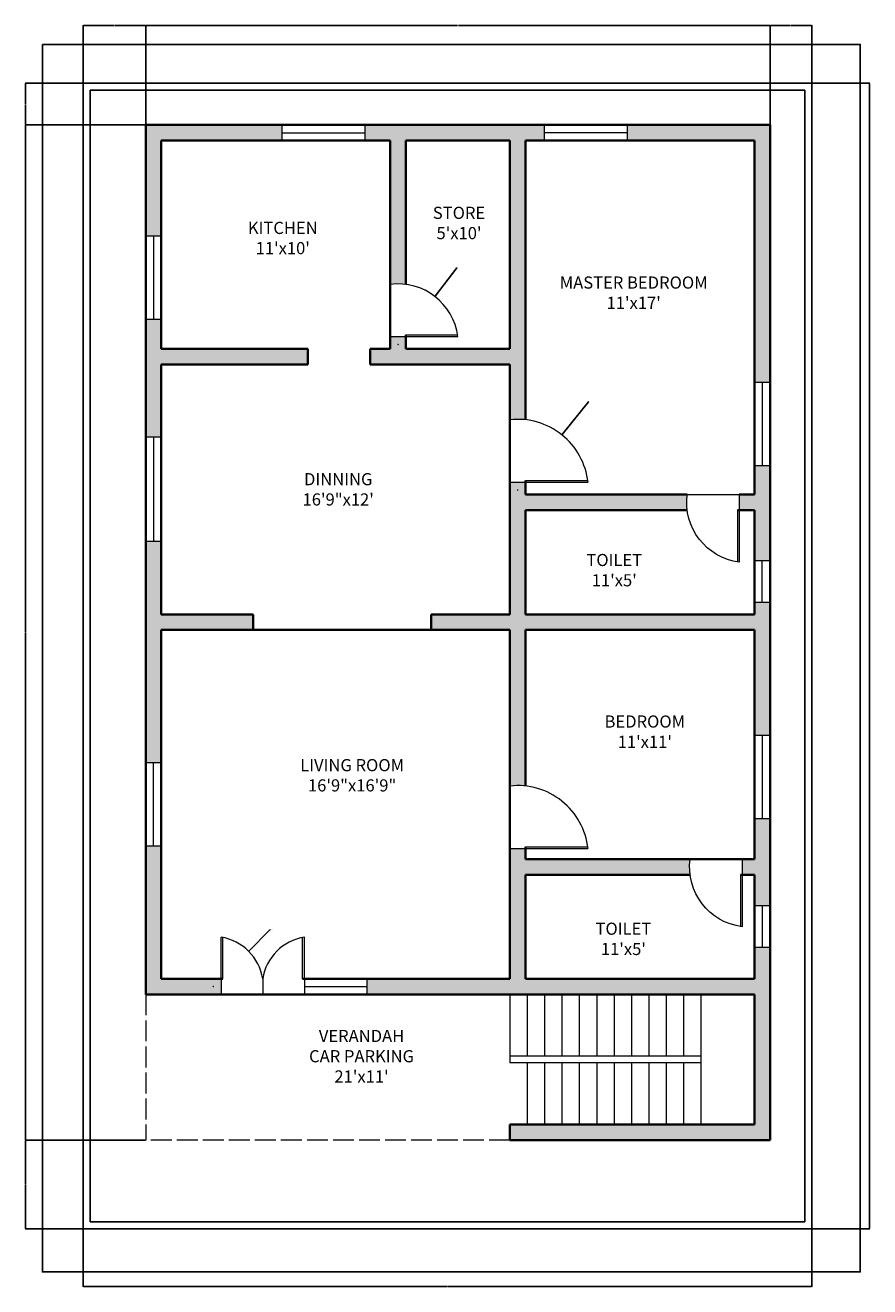
# Model space of a CAD drawing. Units: inches. Extents: x 4948 to 20975, y 6797 to 20508.
# Tile 1 of 5: x 4948 to 5435, y 6797 to 7524. Entities that reach past the tile are written whole.
import ezdxf

# ---------------------------------------------------------------- set-up
doc = ezdxf.new("R2010")
doc.units = ezdxf.units.IN
doc.linetypes.add('ACAD_ISO02W100', pattern=[15, 12, -3])
for name, color, linetype, lineweight in [('A-ANNO-DIMS', 2, 'Continuous', 18), ('A-ANNO-TTLB', 7, 'Continuous', 25), ('A-AREA-IDEN', 7, 'Continuous', 25), ('A-DOOR', 3, 'Continuous', 18), ('A-FLOR-OVHD', 8, 'ACAD_ISO02W100', 18), ('A-FLOR-STRS', 7, 'Continuous', 18), ('A-GLAZ', 4, 'Continuous', 18), ('A-WALL', 7, 'Continuous', 35), ('C-PROP', 7, 'Continuous', 25)]:
    doc.layers.add(name, color=color, linetype=linetype, lineweight=lineweight)
doc.layers.add('A-WALL-PATT', color=18, linetype='Continuous', lineweight=13, true_color=0x000000)
doc.styles.get("Standard").update_dxf_attribs({"font": 'times.ttf'})
doc.dimstyles.get("Standard").update_dxf_attribs({"dimtxt": 0.18, "dimasz": 0.18, "dimexe": 0.18, "dimexo": 0.0625, "dimgap": 0.09, "dimtad": 0, "dimtih": 1, "dimtoh": 1, "dimdec": 4, "dimzin": 0, "dimdsep": 46, "dimtxsty": 'Standard', "dimcen": 0.09, "dimadec": 0, "dimazin": 0, "dimtfac": 1, "dimtdec": 4, "dimtofl": 0, "dimtmove": 0, "dimatfit": 3, "dimfxl": 1, "dimtolj": 1, "dimtzin": 0, "dimarcsym": 0})

# ---------------------------------------------------------------- blocks, each defined once
blk = doc.blocks.new('DOOR-SINGLE-36IN')
for p, q in [((9, 1), (45, 1)), ((0, 0), (9, 0)), ((9, 0), (45, 0))]:
    blk.add_line(p, q)
blk.add_arc((4.5, -4.5), 40.75, 6.34019, 96.34019)
blk = doc.blocks.new('DOOR-SINGLE-30IN')
for p, q in [((0, 0), (9, 0)), ((9, 1), (39, 1)), ((9, 0), (39, 0))]:
    blk.add_line(p, q)
blk.add_arc((4.5, -4.5), 34.79, 7.43141, 97.43141)
blk = doc.blocks.new('DOOR-DOUBLE-48IN')
for p, q in [((0, 9), (0, 33)), ((1, 9), (1, 33)), ((47, 9), (47, 33)), ((48, 9), (48, 33)), ((0, 9), (0, 0)), ((24, 9), (24, 0)), ((48, 9), (48, 0))]:
    blk.add_line(p, q)
for centre, start, end in [((-4.5, 4.5), 8.97263, 81.02737), ((52.5, 4.5), 98.97263, 171.02737)]:
    blk.add_arc(centre, 28.85, start, end)
blk = doc.blocks.new('WIN-48IN')
for p, q in [((0, 0), (0, 9)), ((48, 0), (48, 9)), ((0, 4.5), (48, 4.5))]:
    blk.add_line(p, q)
blk = doc.blocks.new('WIN-24IN')
for p, q in [((0, 24), (9, 24)), ((4.5, 0), (4.5, 24)), ((0, 0), (9, 0))]:
    blk.add_line(p, q)
blk = doc.blocks.new('WIN-SIDELIGHT-36IN')
for p, q in [((36, 9), (36, 0)), ((0, 4.5), (36, 4.5))]:
    blk.add_line(p, q)
blk = doc.blocks.new('WIN-60IN')
for p, q in [((9, 60), (0, 60)), ((4.5, 60), (4.5, 0)), ((9, 0), (0, 0))]:
    blk.add_line(p, q)
blk = doc.blocks.new('STAIR-RETURN-110IN')
for p, q in [((0, 75), (0, 35.5)), ((10, 75), (10, 39.5)), ((20, 75), (20, 39.5)), ((30, 75), (30, 39.5)), ((40, 75), (40, 39.5)), ((50, 75), (50, 39.5)), ((60, 75), (60, 39.5)), ((70, 75), (70, 39.5)), ((80, 75), (80, 39.5)), ((90, 75), (90, 39.5)), ((100, 75), (100, 39.5)), ((110, 75), (110, 0)), ((110, 39.5), (0, 39.5)), ((110, 35.5), (0, 35.5)), ((10, 35.5), (10, 0)), ((20, 35.5), (20, 0)), ((30, 35.5), (30, 0)), ((40, 35.5), (40, 0)), ((50, 35.5), (50, 0)), ((60, 35.5), (60, 0)), ((70, 35.5), (70, 0)), ((80, 35.5), (80, 0)), ((90, 35.5), (90, 0)), ((100, 35.5), (100, 0))]:
    blk.add_line(p, q)
blk = doc.blocks.new('*D25')
at = {"layer": 'A-ANNO-DIMS', "color": 0, "lineweight": -2, "transparency": 16777216}
for p, q in [((4981.22, 6830.38), (4981.22, 6797.01)), ((5401.22, 6830.38), (5401.22, 6797.01)), ((4981.4, 6797.19), (5190.94, 6797.19)), ((5401.04, 6797.19), (5191.5, 6797.19))]:
    blk.add_line(p, q, dxfattribs=at)
at = {"layer": 'A-ANNO-DIMS', "color": 0, "transparency": 16777216}
for points in [[(4981.4, 6797.22), (4981.4, 6797.16), (4981.22, 6797.19)], [(5401.04, 6797.22), (5401.04, 6797.16), (5401.22, 6797.19)]]:
    blk.add_solid(points, dxfattribs=at)
at = {"layer": 'Defpoints', "color": 0, "transparency": 16777216}
for p in [(4981.22, 6830.44), (5401.22, 6830.44), (5401.22, 6797.19)]:
    blk.add_point(p, dxfattribs=at)
at = {"layer": 'A-ANNO-DIMS', "color": 0, "transparency": 16777216, "insert": (5191.22, 6797.19), "char_height": 0.18, "attachment_point": 5}
blk.add_mtext('\\A1;420', dxfattribs=at)
blk = doc.blocks.new('*D26')
at = {"layer": 'A-ANNO-DIMS', "color": 0, "lineweight": -2, "transparency": 16777216}
for p, q in [((5401.28, 7490.44), (5434.65, 7490.44)), ((5434.47, 7490.26), (5434.47, 7160.63)), ((5434.47, 6830.62), (5434.47, 7160.26)), ((5401.28, 6830.44), (5434.65, 6830.44))]:
    blk.add_line(p, q, dxfattribs=at)
at = {"layer": 'A-ANNO-DIMS', "color": 0, "transparency": 16777216}
for points in [[(5434.44, 7490.26), (5434.5, 7490.26), (5434.47, 7490.44)], [(5434.44, 6830.62), (5434.5, 6830.62), (5434.47, 6830.44)]]:
    blk.add_solid(points, dxfattribs=at)
at = {"layer": 'Defpoints', "color": 0, "transparency": 16777216}
for p in [(5401.22, 7490.44), (5434.47, 7490.44), (5401.22, 6830.44)]:
    blk.add_point(p, dxfattribs=at)
at = {"layer": 'A-ANNO-DIMS', "color": 0, "transparency": 16777216, "insert": (5434.47, 7160.44), "char_height": 0.18, "attachment_point": 5}
blk.add_mtext('\\A1;660', dxfattribs=at)
blk = doc.blocks.new('*D27')
at = {"layer": 'A-ANNO-DIMS', "color": 0, "lineweight": -2, "transparency": 16777216}
for p, q in [((5017.22, 7466.51), (5017.22, 7523.87)), ((5017.4, 7523.69), (5196.94, 7523.69)), ((5377.04, 7523.69), (5197.5, 7523.69)), ((5377.22, 7466.51), (5377.22, 7523.87))]:
    blk.add_line(p, q, dxfattribs=at)
at = {"layer": 'A-ANNO-DIMS', "color": 0, "transparency": 16777216}
for points in [[(5017.4, 7523.72), (5017.4, 7523.66), (5017.22, 7523.69)], [(5377.04, 7523.72), (5377.04, 7523.66), (5377.22, 7523.69)]]:
    blk.add_solid(points, dxfattribs=at)
at = {"layer": 'Defpoints', "color": 0, "transparency": 16777216}
for p in [(5377.22, 7523.69), (5017.22, 7466.44), (5377.22, 7466.44)]:
    blk.add_point(p, dxfattribs=at)
at = {"layer": 'A-ANNO-DIMS', "color": 0, "transparency": 16777216, "insert": (5197.22, 7523.69), "char_height": 0.18, "attachment_point": 5}
blk.add_mtext('\\A1;360', dxfattribs=at)
blk = doc.blocks.new('*D28')
at = {"layer": 'A-ANNO-DIMS', "color": 0, "lineweight": -2, "transparency": 16777216}
for p, q in [((5017.16, 7466.44), (4947.79, 7466.44)), ((4947.97, 7466.26), (4947.97, 7174.13)), ((4947.97, 6881.62), (4947.97, 7173.76)), ((5017.16, 6881.44), (4947.79, 6881.44))]:
    blk.add_line(p, q, dxfattribs=at)
at = {"layer": 'A-ANNO-DIMS', "color": 0, "transparency": 16777216}
for points in [[(4947.94, 7466.26), (4948, 7466.26), (4947.97, 7466.44)], [(4947.94, 6881.62), (4948, 6881.62), (4947.97, 6881.44)]]:
    blk.add_solid(points, dxfattribs=at)
at = {"layer": 'Defpoints', "color": 0, "transparency": 16777216}
for p in [(4947.97, 7466.44), (5017.22, 7466.44), (5017.22, 6881.44)]:
    blk.add_point(p, dxfattribs=at)
at = {"layer": 'A-ANNO-DIMS', "color": 0, "transparency": 16777216, "insert": (4947.97, 7173.94), "char_height": 0.18, "attachment_point": 5}
blk.add_mtext('\\A1;585', dxfattribs=at)
blk = doc.blocks.new('*D29')
at = {"layer": 'A-ANNO-DIMS', "color": 0, "lineweight": -2, "transparency": 16777216}
for p, q in [((4981.22, 7490.51), (4981.22, 7523.87)), ((4981.4, 7523.69), (4999.01, 7523.69)), ((5017.04, 7523.69), (4999.43, 7523.69)), ((5017.22, 7466.51), (5017.22, 7523.87))]:
    blk.add_line(p, q, dxfattribs=at)
at = {"layer": 'A-ANNO-DIMS', "color": 0, "transparency": 16777216}
for points in [[(4981.4, 7523.72), (4981.4, 7523.66), (4981.22, 7523.69)], [(5017.04, 7523.72), (5017.04, 7523.66), (5017.22, 7523.69)]]:
    blk.add_solid(points, dxfattribs=at)
at = {"layer": 'Defpoints', "color": 0, "transparency": 16777216}
for p in [(5017.22, 7523.69), (4981.22, 7490.44), (5017.22, 7466.44)]:
    blk.add_point(p, dxfattribs=at)
at = {"layer": 'A-ANNO-DIMS', "color": 0, "transparency": 16777216, "insert": (4999.22, 7523.69), "char_height": 0.18, "attachment_point": 5}
blk.add_mtext('\\A1;36', dxfattribs=at)
blk = doc.blocks.new('*D30')
at = {"layer": 'A-ANNO-DIMS', "color": 0, "lineweight": -2, "transparency": 16777216}
for p, q in [((5377.22, 7466.51), (5377.22, 7523.87)), ((5377.4, 7523.69), (5389, 7523.69)), ((5401.04, 7523.69), (5389.43, 7523.69)), ((5401.22, 7490.51), (5401.22, 7523.87))]:
    blk.add_line(p, q, dxfattribs=at)
at = {"layer": 'A-ANNO-DIMS', "color": 0, "transparency": 16777216}
for points in [[(5377.4, 7523.72), (5377.4, 7523.66), (5377.22, 7523.69)], [(5401.04, 7523.72), (5401.04, 7523.66), (5401.22, 7523.69)]]:
    blk.add_solid(points, dxfattribs=at)
at = {"layer": 'Defpoints', "color": 0, "transparency": 16777216}
for p in [(5401.22, 7523.69), (5401.22, 7490.44), (5377.22, 7466.44)]:
    blk.add_point(p, dxfattribs=at)
at = {"layer": 'A-ANNO-DIMS', "color": 0, "transparency": 16777216, "insert": (5389.22, 7523.69), "char_height": 0.18, "attachment_point": 5}
blk.add_mtext('\\A1;24', dxfattribs=at)
blk = doc.blocks.new('*D31')
at = {"layer": 'A-ANNO-DIMS', "color": 0, "lineweight": -2, "transparency": 16777216}
for p, q in [((4981.156446, 7490.444038), (4947.788946, 7490.444038)), ((4947.968946, 7490.264038), (4947.968946, 7478.624038)), ((4947.968946, 7466.624038), (4947.968946, 7478.264038)), ((5017.156446, 7466.444038), (4947.788946, 7466.444038))]:
    blk.add_line(p, q, dxfattribs=at)
at = {"layer": 'A-ANNO-DIMS', "color": 0, "transparency": 16777216}
for points in [[(4947.938946, 7490.264038), (4947.998946, 7490.264038), (4947.968946, 7490.444038)], [(4947.938946, 7466.624038), (4947.998946, 7466.624038), (4947.968946, 7466.444038)]]:
    blk.add_solid(points, dxfattribs=at)
at = {"layer": 'Defpoints', "color": 0, "transparency": 16777216}
for p in [(4981.218946, 7490.444038), (4947.968946, 7466.444038), (5017.218946, 7466.444038)]:
    blk.add_point(p, dxfattribs=at)
at = {"layer": 'A-ANNO-DIMS', "color": 0, "transparency": 16777216, "insert": (4947.968946, 7478.444038), "char_height": 0.18, "attachment_point": 5}
blk.add_mtext('\\A1;24', dxfattribs=at)
blk = doc.blocks.new('*D32')
at = {"layer": 'A-ANNO-DIMS', "color": 0, "lineweight": -2, "transparency": 16777216}
for p, q in [((5017.16, 6881.44), (4947.79, 6881.44)), ((4947.97, 6881.26), (4947.97, 6856.13)), ((4947.97, 6830.62), (4947.97, 6855.76)), ((4981.16, 6830.44), (4947.79, 6830.44))]:
    blk.add_line(p, q, dxfattribs=at)
at = {"layer": 'A-ANNO-DIMS', "color": 0, "transparency": 16777216}
for points in [[(4947.94, 6881.26), (4948, 6881.26), (4947.97, 6881.44)], [(4947.94, 6830.62), (4948, 6830.62), (4947.97, 6830.44)]]:
    blk.add_solid(points, dxfattribs=at)
at = {"layer": 'Defpoints', "color": 0, "transparency": 16777216}
for p in [(4947.97, 6881.44), (5017.22, 6881.44), (4981.22, 6830.44)]:
    blk.add_point(p, dxfattribs=at)
at = {"layer": 'A-ANNO-DIMS', "color": 0, "transparency": 16777216, "insert": (4947.97, 6855.94), "char_height": 0.18, "attachment_point": 5}
blk.add_mtext('\\A1;51', dxfattribs=at)
blk = doc.blocks.new('*D87')
at = {"layer": 'A-ANNO-DIMS', "color": 0, "lineweight": -2, "transparency": 16777216}
for p, q in [((5272.45, 7306.96), (5257.29, 7288.01)), ((5272.63, 7306.96), (5272.45, 7306.96)), ((5231.63, 7256.05), (5231.81, 7256.05)), ((5231.72, 7255.96), (5231.72, 7256.14))]:
    blk.add_line(p, q, dxfattribs=at)
at = {"layer": 'A-ANNO-DIMS', "color": 0, "transparency": 16777216}
blk.add_solid([(5257.26, 7288.03), (5257.31, 7287.99), (5257.18, 7287.87)], dxfattribs=at)
at = {"layer": 'Defpoints', "color": 0, "transparency": 16777216}
for p in [(5257.18, 7287.87), (5231.72, 7256.05)]:
    blk.add_point(p, dxfattribs=at)
at = {"layer": 'A-ANNO-DIMS', "color": 0, "transparency": 16777216, "insert": (5273.29, 7306.96), "char_height": 0.18, "attachment_point": 5}
blk.add_mtext('\\A1;2X R40.75', dxfattribs=at)
blk = doc.blocks.new('*D88')
at = {"layer": 'A-ANNO-DIMS', "color": 0, "lineweight": -2, "transparency": 16777216}
for p, q in [((5196.66, 7384.13), (5184.04, 7367.73)), ((5196.84, 7384.13), (5196.66, 7384.13)), ((5162.63, 7340.01), (5162.81, 7340.01)), ((5162.72, 7339.92), (5162.72, 7340.1))]:
    blk.add_line(p, q, dxfattribs=at)
at = {"layer": 'A-ANNO-DIMS', "color": 0, "transparency": 16777216}
blk.add_solid([(5184.02, 7367.75), (5184.07, 7367.71), (5183.93, 7367.59)], dxfattribs=at)
at = {"layer": 'Defpoints', "color": 0, "transparency": 16777216}
for p in [(5183.93, 7367.59), (5162.72, 7340.01)]:
    blk.add_point(p, dxfattribs=at)
at = {"layer": 'A-ANNO-DIMS', "color": 0, "transparency": 16777216, "insert": (5197.31, 7384.13), "char_height": 0.18, "attachment_point": 5}
blk.add_mtext('\\A1;R34.79', dxfattribs=at)
blk = doc.blocks.new('*D89')
at = {"layer": 'A-ANNO-DIMS', "color": 0, "lineweight": -2, "transparency": 16777216}
for p, q in [((5088.83, 7002.59), (5076.71, 6990.47)), ((5089.01, 7002.59), (5088.83, 7002.59)), ((5056.09, 6969.94), (5056.27, 6969.94)), ((5056.18, 6969.85), (5056.18, 6970.03))]:
    blk.add_line(p, q, dxfattribs=at)
at = {"layer": 'A-ANNO-DIMS', "color": 0, "transparency": 16777216}
blk.add_solid([(5076.69, 6990.49), (5076.73, 6990.45), (5076.58, 6990.35)], dxfattribs=at)
at = {"layer": 'Defpoints', "color": 0, "transparency": 16777216}
for p in [(5076.58, 6990.35), (5056.18, 6969.94)]:
    blk.add_point(p, dxfattribs=at)
at = {"layer": 'A-ANNO-DIMS', "color": 0, "transparency": 16777216, "insert": (5089.73, 7002.59), "char_height": 0.18, "attachment_point": 5}
blk.add_mtext('\\A1;2X R28.853', dxfattribs=at)

msp = doc.modelspace()

# ---------------------------------------------------------------- hatches: boundary and pattern name
at = {"layer": 'A-WALL-PATT'}
h = msp.add_hatch(color=256, dxfattribs=at)
h.dxf.hatch_style = 1
h.paths.add_polyline_path([(5095.8403, 7466.444), (5017.2189, 7466.444), (5017.2189, 7402.5352), (5026.2189, 7402.5352), (5026.2189, 7457.444), (5095.8403, 7457.444)])
h.paths.add_polyline_path([(5246.8789, 7466.444), (5143.8403, 7466.444), (5143.8403, 7457.444), (5158.2189, 7457.444), (5158.2189, 7374.5094, -0.06494234), (5167.2189, 7374.5094), (5167.2189, 7457.444), (5227.2189, 7457.444), (5227.2189, 7337.444), (5167.2189, 7337.444), (5167.2189, 7344.5094), (5158.2189, 7344.5094), (5158.2189, 7337.444), (5146.6872, 7337.444), (5146.6872, 7328.444), (5227.2189, 7328.444), (5227.2189, 7296.5526, -0.05538514), (5236.2189, 7296.5526), (5236.2189, 7328.444), (5236.2189, 7457.444), (5246.8789, 7457.444)])
h.paths.add_polyline_path([(5377.2189, 7466.444), (5294.8789, 7466.444), (5294.8789, 7457.444), (5368.2189, 7457.444), (5368.2189, 7318.1488), (5377.2189, 7318.1488)])
h.paths.add_polyline_path([(5026.2189, 7328.444), (5110.6872, 7328.444), (5110.6872, 7337.444), (5026.2189, 7337.444), (5026.2189, 7354.5352), (5017.2189, 7354.5352), (5017.2189, 7286.444), (5026.2189, 7286.444)])
h.paths.add_polyline_path([(5377.2189, 7191.5422), (5368.2189, 7191.5422), (5368.2189, 7184.444), (5236.2189, 7184.444), (5236.2189, 7244.444), (5329.4566, 7244.444, -0.06494234), (5329.4566, 7253.444), (5236.2189, 7253.444), (5236.2189, 7260.5526), (5227.2189, 7260.5526), (5227.2189, 7244.444), (5227.2189, 7184.444), (5181.8226, 7184.444), (5181.8226, 7175.444), (5227.2189, 7175.444), (5227.2189, 7085.5219, -0.05538514), (5236.2189, 7085.5219), (5236.2189, 7175.444), (5368.2189, 7175.444), (5368.2189, 7114.8955), (5377.2189, 7114.8955)])
h.paths.add_polyline_path([(5377.2189, 7270.1488), (5368.2189, 7270.1488), (5368.2189, 7253.444), (5359.4566, 7253.444), (5359.4566, 7244.444), (5368.2189, 7244.444), (5368.2189, 7215.5422), (5377.2189, 7215.5422)])
h.paths.add_polyline_path([(5377.2189, 7066.8955), (5368.2189, 7066.8955), (5368.2189, 7043.444), (5361.0558, 7043.444), (5361.0558, 7034.444), (5368.2189, 7034.444), (5368.2189, 7016.444), (5377.2189, 7016.444)])
h.paths.add_polyline_path([(5377.2189, 6992.444), (5368.2189, 6992.444), (5368.2189, 6974.444), (5236.2189, 6974.444), (5236.2189, 7034.444), (5331.0558, 7034.444, -0.06494234), (5331.0558, 7043.444), (5236.2189, 7043.444), (5236.2189, 7049.5219), (5227.2189, 7049.5219), (5227.2189, 6974.444), (5144.6817, 6974.444), (5144.6817, 6965.444), (5227.2189, 6965.444), (5236.2189, 6965.444), (5368.2189, 6965.444), (5368.2189, 6890.444), (5227.2189, 6890.444), (5227.2189, 6881.444), (5377.2189, 6881.444)])
h.paths.add_polyline_path([(5060.6817, 6974.444), (5026.2189, 6974.444), (5026.2189, 7050.944), (5017.2189, 7050.944), (5017.2189, 6965.444), (5026.2189, 6965.444), (5060.6817, 6965.444)])
h.paths.add_polyline_path([(5026.2189, 7175.444), (5079.1853, 7175.444), (5079.1853, 7184.444), (5026.2189, 7184.444), (5026.2189, 7226.444), (5017.2189, 7226.444), (5017.2189, 7098.944), (5026.2189, 7098.944)])

# ---------------------------------------------------------------- linework, layer by layer
at = {"layer": 'A-ANNO-TTLB'}
msp.add_lwpolyline([(4957.7293, 7512.8595), (5429.1896, 7512.8595), (5429.1896, 6805.5342), (4957.7293, 6805.5342)], close=True, dxfattribs=at)
at = {"layer": 'A-DOOR'}
msp.add_line((5329.4566, 7253.444), (5359.4566, 7253.444), dxfattribs=at)
at = {"layer": 'A-FLOR-OVHD'}
for p in [(5017.2189, 6965.444), (5227.2189, 6881.444)]:
    msp.add_line(p, (5017.2189, 6881.444), dxfattribs=at)
at = {"layer": 'A-WALL'}
for p, q in [((5017.2189, 6965.444), (5017.2189, 7466.444)), ((5017.2189, 7466.444), (5377.2189, 7466.444)), ((5377.2189, 7466.444), (5377.2189, 6881.444)), ((5026.2189, 7457.444), (5158.2189, 7457.444)), ((5026.2189, 7337.444), (5026.2189, 7457.444)), ((5158.2189, 7337.444), (5158.2189, 7457.444)), ((5167.2189, 7457.444), (5227.2189, 7457.444)), ((5167.2189, 7374.5094), (5167.2189, 7457.444)), ((5227.2189, 7337.444), (5227.2189, 7457.444)), ((5236.2189, 7328.444), (5236.2189, 7457.444)), ((5236.2189, 7457.444), (5368.2189, 7457.444)), ((5368.2189, 7457.444), (5368.2189, 7253.444)), ((5167.2189, 7337.444), (5167.2189, 7345.5094)), ((5026.2189, 7337.444), (5110.6872, 7337.444)), ((5110.6872, 7337.444), (5110.6872, 7328.444)), ((5146.6872, 7337.444), (5146.6872, 7328.444)), ((5146.6872, 7337.444), (5158.2189, 7337.444)), ((5167.2189, 7337.444), (5227.2189, 7337.444)), ((5026.2189, 7328.444), (5110.6872, 7328.444)), ((5026.2189, 7184.444), (5026.2189, 7328.444)), ((5146.6872, 7328.444), (5227.2189, 7328.444)), ((5227.2189, 7328.444), (5227.2189, 7244.444)), ((5236.2189, 7328.444), (5236.2189, 7296.5526)), ((5236.2189, 7261.5526), (5236.2189, 7253.444)), ((5236.2189, 7253.444), (5329.4566, 7253.444)), ((5359.4566, 7253.444), (5368.2189, 7253.444)), ((5227.2189, 7244.444), (5227.2189, 7184.444)), ((5236.2189, 7244.444), (5329.4566, 7244.444)), ((5236.2189, 7244.444), (5236.2189, 7184.444)), ((5358.4566, 7244.444), (5368.2189, 7244.444)), ((5368.2189, 7244.444), (5368.2189, 7184.444)), ((5026.2189, 7184.444), (5079.1853, 7184.444)), ((5079.1853, 7175.444), (5079.1853, 7184.444)), ((5181.8226, 7175.444), (5181.8226, 7184.444)), ((5181.8226, 7184.444), (5227.2189, 7184.444)), ((5236.2189, 7184.444), (5368.2189, 7184.444)), ((5026.2189, 7175.444), (5079.1853, 7175.444)), ((5026.2189, 6974.444), (5026.2189, 7175.444)), ((5079.1853, 7175.444), (5181.8226, 7175.444)), ((5181.8226, 7175.444), (5227.2189, 7175.444)), ((5227.2189, 7175.444), (5227.2189, 6974.444)), ((5236.2189, 7175.444), (5236.2189, 7085.5219)), ((5236.2189, 7175.444), (5368.2189, 7175.444)), ((5368.2189, 7175.444), (5368.2189, 7043.444)), ((5236.2189, 7050.5219), (5236.2189, 7043.444)), ((5236.2189, 7043.444), (5368.2189, 7043.444)), ((5236.2189, 7034.444), (5331.0558, 7034.444)), ((5236.2189, 7034.444), (5236.2189, 6974.444)), ((5360.0558, 7034.444), (5368.2189, 7034.444)), ((5368.2189, 7034.444), (5368.2189, 6974.444)), ((5026.2189, 6974.444), (5061.6817, 6974.444)), ((5107.6817, 6974.444), (5227.2189, 6974.444)), ((5236.2189, 6974.444), (5368.2189, 6974.444)), ((5026.2189, 6965.444), (5017.2189, 6965.444)), ((5026.2189, 6965.444), (5227.2189, 6965.444)), ((5227.2189, 6965.444), (5236.2189, 6965.444)), ((5236.2189, 6965.444), (5368.2189, 6965.444)), ((5368.2189, 6965.444), (5368.2189, 6890.444)), ((5368.2189, 6890.444), (5227.2189, 6890.444)), ((5227.2189, 6890.444), (5227.2189, 6881.444)), ((5377.2189, 6881.444), (5227.2189, 6881.444))]:
    msp.add_line(p, q, dxfattribs=at)
at = {"layer": 'C-PROP'}
for p, q in [((4981.2189, 7490.444), (5401.2189, 7490.444)), ((4981.2189, 6830.444), (4981.2189, 7490.444)), ((5401.2189, 7490.444), (5401.2189, 6830.444)), ((4985.2189, 7486.444), (5397.2189, 7486.444)), ((4985.2189, 6834.444), (4985.2189, 7486.444)), ((5397.2189, 7486.444), (5397.2189, 6834.444)), ((5397.2189, 6834.444), (4985.2189, 6834.444)), ((5401.2189, 6830.444), (4981.2189, 6830.444))]:
    msp.add_line(p, q, dxfattribs=at)

# ---------------------------------------------------------------- block references
at = {"layer": 'A-DOOR'}
for name, p in [('DOOR-SINGLE-30IN', (5158.219, 7344.509)), ('DOOR-SINGLE-36IN', (5227.219, 7260.553)), ('DOOR-SINGLE-36IN', (5227.219, 7049.5222)), ('DOOR-DOUBLE-48IN', (5060.682, 6965.444))]:
    msp.add_blockref(name, p, dxfattribs=at)
at = {"layer": 'A-DOOR', "extrusion": (0, 0, -1), "zscale": -1}
for p, rotation in [((-5359.4571, 7253.444), 269.9999999999948), ((-5361.0562, 7043.444), 269.9999999999951)]:
    msp.add_blockref('DOOR-SINGLE-30IN', p, dxfattribs=dict(at, rotation=rotation))
at = {"layer": 'A-FLOR-STRS'}
msp.add_blockref('STAIR-RETURN-110IN', (5227.219, 6890.444), dxfattribs=at)
at = {"layer": 'A-GLAZ'}
for name, p in [('WIN-48IN', (5095.84, 7457.444)), ('WIN-60IN', (5017.219, 7226.444)), ('WIN-24IN', (5368.219, 7191.542)), ('WIN-SIDELIGHT-36IN', (5108.682, 6965.444))]:
    msp.add_blockref(name, p, dxfattribs=at)
for name, p, rotation in [('WIN-48IN', (5294.8792, 7466.4441), 180), ('WIN-48IN', (5017.2189, 7402.5355), 269.999999999995), ('WIN-48IN', (5368.2189, 7318.1491), 269.9999999999816), ('WIN-48IN', (5368.2189, 7114.8958), 269.9999999999971), ('WIN-48IN', (5026.219, 7050.9437), 89.99999999999083), ('WIN-24IN', (5377.2189, 7016.4442), 180)]:
    msp.add_blockref(name, p, dxfattribs=dict(at, rotation=rotation))

# ---------------------------------------------------------------- texts
at = {"layer": 'A-AREA-IDEN', "char_height": 7, "attachment_point": 1}
for s, width, insert in [("\\pxqc;{\\fTimes New Roman|b1|i0|c0|p18;STORE\\P5'x10'}", 45.669043, (5175.0326, 7419.2695)), ("\\pxqc;{\\fTimes New Roman|b1|i0|c0|p18;KITCHEN\\P11'x10'}", 91.794797, (5050.3561, 7410.5979)), ("\\pxqc;{\\fTimes New Roman|b1|i0|c0|p18;MASTER BEDROOM 11'x17'}", 108.235638, (5244.4496, 7379.1063)), ('\\pxqc;{\\fTimes New Roman|b1|i0|c0|p18;DINNING\\P16\'9"x12\'}', 128.330031, (5064.0518, 7265.8125)), ("\\pxqc;{\\fTimes New Roman|b1|i0|c0|p18;TOILET\\P11'x5'}", 86.771181, (5243.9879, 7219.2596)), ("\\pxqc;{\\fTimes New Roman|b1|i0|c0|p18;BEDROOM\\P11'x11'}", 109.747903, (5250.1091, 7126.191)), ('\\pxqc;{\\fTimes New Roman|b1|i0|c0|p18;LIVING ROOM\\P16\'9"x16\'9"}', 113.406157, (5079.5425, 7101.0564)), ("\\pxqc;{\\fTimes New Roman|b1|i0|c0|p18;TOILET\\P11'x5'}", 85.969216, (5249.6482, 7006.8141)), ("\\pxqc;{\\fTimes New Roman|b1|i0|c0|p18;VERANDAH\\PCAR PARKING\\P21'x11'}", 117.979027, (5082.671, 6945.0119))]:
    msp.add_mtext_dynamic_manual_height_columns(s, width=width, gutter_width=12.5, heights=[0], dxfattribs=dict(at, insert=insert))

# ---------------------------------------------------------------- dimensions: what is measured, and where the dimension line sits
at = {"layer": 'A-ANNO-DIMS'}
for base, p1, p2, picture, middle in [((5017.2189, 7523.694), (4981.2189, 7490.444), (5017.2189, 7466.444), '*D29', (4999.2189, 7523.694)), ((5377.2189, 7523.694), (5017.2189, 7466.444), (5377.2189, 7466.444), '*D27', (5197.2189, 7523.694)), ((5401.2189, 7523.694), (5377.2189, 7466.444), (5401.2189, 7490.444), '*D30', (5389.2189, 7523.694)), ((5401.2189, 6797.194), (4981.2189, 6830.444), (5401.2189, 6830.444), '*D25', (5191.2189, 6797.194))]:
    dim = msp.add_linear_dim(base=base, p1=p1, p2=p2, dimstyle='Standard', override={"dimdec": 0, "dimlfac": 1, "dimrnd": 0, "dimzin": 0, "dimdsep": 46, "dimlunit": 2}, dxfattribs=at)
    dim.commit()
    dim.dimension.update_dxf_attribs({"geometry": picture, "text_midpoint": middle})
for base, p1, p2, picture, middle in [((4947.9689, 7466.444), (4981.2189, 7490.444), (5017.2189, 7466.444), '*D31', (4947.9689, 7478.444)), ((5434.4689, 7490.444), (5401.2189, 6830.444), (5401.2189, 7490.444), '*D26', (5434.4689, 7160.444)), ((4947.9689, 7466.444), (5017.2189, 6881.444), (5017.2189, 7466.444), '*D28', (4947.9689, 7173.944)), ((4947.9689, 6881.444), (4981.2189, 6830.444), (5017.2189, 6881.444), '*D32', (4947.9689, 6855.944))]:
    dim = msp.add_linear_dim(base=base, p1=p1, p2=p2, angle=90, dimstyle='Standard', override={"dimdec": 0, "dimlfac": 1, "dimrnd": 0, "dimzin": 0, "dimdsep": 46, "dimlunit": 2}, dxfattribs=at)
    dim.commit()
    dim.dimension.update_dxf_attribs({"geometry": picture, "text_midpoint": middle})
dim = msp.add_radius_dim(center=(5162.7189, 7340.0094), mpoint=(5183.9319, 7367.5868), dimstyle='Standard', override={"dimdec": 2, "dimlfac": 1, "dimrnd": 0, "dimzin": 0, "dimdsep": 46, "dimlunit": 2}, dxfattribs=at)
dim.commit()
dim.dimension.update_dxf_attribs({"geometry": '*D88', "text_midpoint": (5197.3093, 7384.1333), "dimtype": 164})
for center, mpoint, override, picture, middle in [((5231.7189, 7256.0526), (5257.1751, 7287.8722), {"dimdec": 2, "dimlfac": 1, "dimrnd": 0, "dimzin": 0, "dimdsep": 46, "dimlunit": 2}, '*D87', (5273.2905, 7306.9639)), ((5056.1817, 6969.944), (5076.5841, 6990.3461), {"dimdec": 3, "dimlfac": 1, "dimrnd": 0, "dimzin": 0, "dimdsep": 46, "dimlunit": 2}, '*D89', (5089.7313, 7002.5873))]:
    dim = msp.add_radius_dim(center=center, mpoint=mpoint, text='2X <>', dimstyle='Standard', override=override, dxfattribs=at)
    dim.commit()
    dim.dimension.update_dxf_attribs({"geometry": picture, "text_midpoint": middle, "dimtype": 164})

doc.saveas('drawing.dxf')
